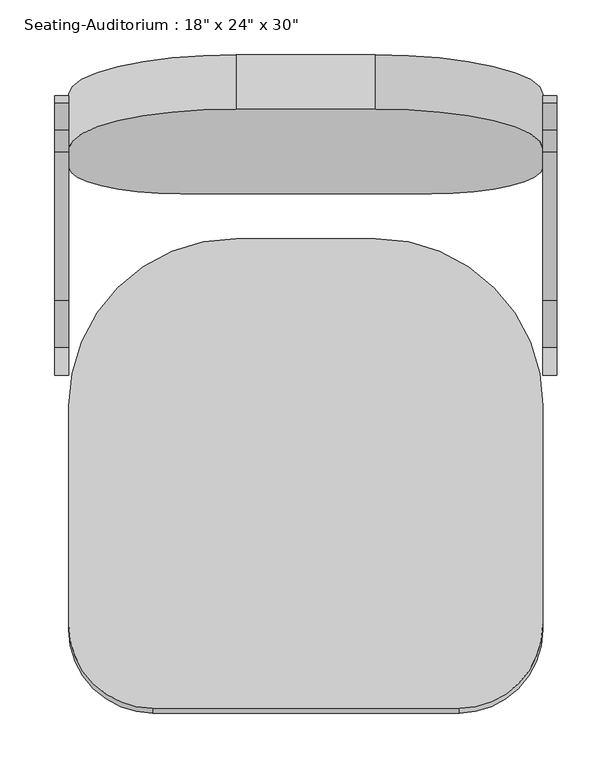
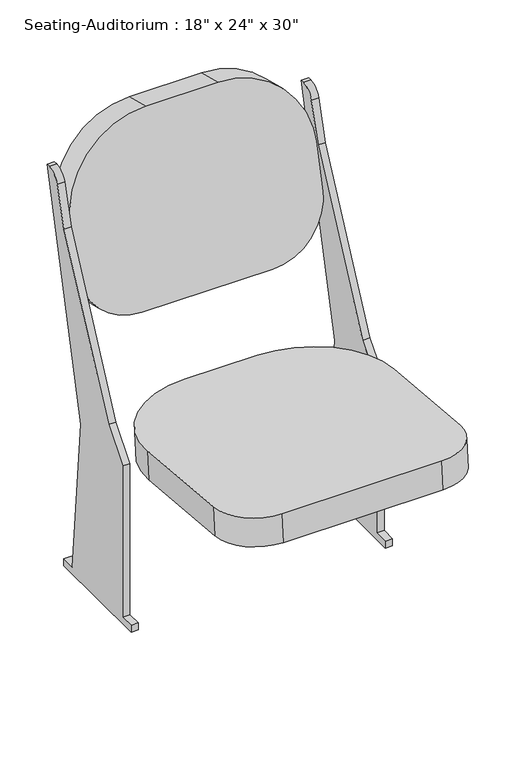
"""IFC4 building model written with IfcOpenShell, lengths in millimetres: furniture geometry."""

from ifc_helpers import new_model, si_unit, point, frame, frame_2d, origin, place, context, project, spatial, polyline, circle_curve, trimmed, segment, composite_curve, outline, extrude, source, transform, mapped, element, save


def furniture_4fdbbe14(model_context):
    return source(origin(), model_context, "Body", "SweptSolid", [
        extrude(outline(composite_curve([segment(polyline([(13.3245902, 12.7), (13.3245902, 0.0), (-189.8754098, 0.0), (-189.8754098, 12.7), (-164.4754098, 12.7), (-164.4754098, 292.1), (-121.8491486, 342.9), (13.3245902, 622.3), (33.4611378, 692.7779166)]), True, "CONTINUOUS"), segment(trimmed(circle_curve(frame_2d((57.883846, 685.8)), 25.4), [point((33.4611378, 692.7779166))], [point((57.883846, 711.2))], False, "CARTESIAN"), True, "CONTINUOUS"), segment(polyline([(57.883846, 711.2), (64.1245902, 711.2), (-37.4754098, 292.1), (-12.0754098, 12.7), (13.3245902, 12.7)]), True, "CONTINUOUS")], self_intersect=False)), frame((376.6278689, 0.0, 0.0), z_axis=(1.0, 0.0, 0.0), x_axis=(0.0, 1.0, 0.0)), (0.0, 0.0, 1.0), 12.7),
        extrude(outline(composite_curve([segment(polyline([(13.3245902, 0.0), (-189.8754098, 0.0), (-189.8754098, 12.7), (-164.4754098, 12.7), (-164.4754098, 292.1), (-121.8491486, 342.9), (13.3245902, 622.3), (33.4611378, 692.7779166)]), True, "CONTINUOUS"), segment(trimmed(circle_curve(frame_2d((57.883846, 685.8)), 25.4), [point((33.4611378, 692.7779166))], [point((57.883846, 711.2))], False, "CARTESIAN"), True, "CONTINUOUS"), segment(polyline([(57.883846, 711.2), (64.1245902, 711.2), (-37.4754098, 292.1), (-12.0754098, 12.7), (13.3245902, 12.7), (13.3245902, 0.0)]), True, "CONTINUOUS")], self_intersect=False)), frame((-67.8721311, 0.0, 0.0), z_axis=(1.0, 0.0, 0.0), x_axis=(0.0, 1.0, 0.0)), (0.0, 0.0, 1.0), 12.7),
        extrude(outline(composite_curve([segment(polyline([(0.0, 0.0), (-279.4, 0.0)]), True, "CONTINUOUS"), segment(trimmed(circle_curve(frame_2d((-279.4, 76.2)), 76.2), [point((-279.4, 0.0))], [point((-355.6, 76.2))], False, "CARTESIAN"), True, "CONTINUOUS"), segment(polyline([(-355.6, 76.2), (-355.6, 276.4123505)]), True, "CONTINUOUS"), segment(trimmed(circle_curve(frame_2d((-203.2, 276.4123505)), 152.4), [point((-355.6, 276.4123505))], [point((-203.2, 428.8123506))], False, "CARTESIAN"), True, "CONTINUOUS"), segment(polyline([(-203.2, 428.8123506), (-76.2, 428.8123506)]), True, "CONTINUOUS"), segment(trimmed(circle_curve(frame_2d((-76.2, 276.4123505)), 152.4), [point((-76.2, 428.8123506))], [point((76.2, 276.4123505))], False, "CARTESIAN"), True, "CONTINUOUS"), segment(polyline([(76.2, 276.4123505), (76.2, 76.2)]), True, "CONTINUOUS"), segment(trimmed(circle_curve(frame_2d((0.0, 76.2)), 76.2), [point((76.2, 76.2))], [point((0.0, 0.0))], False, "CARTESIAN"), True, "CONTINUOUS")], self_intersect=False)), frame((300.4278689, -497.5245173, 321.2380213), z_axis=(0.0, 0.08715574274765496, 0.9961946980917459), x_axis=(1.0, 0.0, 0.0)), (0.0, 0.0, 1.0), 50.8),
        extrude(outline(composite_curve([segment(trimmed(circle_curve(frame_2d((0.0, 152.4)), 152.4), [point((0.0, 0.0))], [point((-152.4, 152.4))], False, "CARTESIAN"), True, "CONTINUOUS"), segment(polyline([(-152.4, 152.4), (-152.4, 224.0588601)]), True, "CONTINUOUS"), segment(trimmed(circle_curve(frame_2d((-50.8, 224.0588601)), 101.6), [point((-152.4, 224.0588601))], [point((-50.8, 325.6588601))], False, "CARTESIAN"), True, "CONTINUOUS"), segment(polyline([(-50.8, 325.6588601), (177.8, 325.6588601)]), True, "CONTINUOUS"), segment(trimmed(circle_curve(frame_2d((177.8, 224.0588601)), 101.6), [point((177.8, 325.6588601))], [point((279.4, 224.0588601))], False, "CARTESIAN"), True, "CONTINUOUS"), segment(polyline([(279.4, 224.0588601), (279.4, 152.4)]), True, "CONTINUOUS"), segment(trimmed(circle_curve(frame_2d((127.0, 152.4)), 152.4), [point((279.4, 152.4))], [point((127.0, 0.0))], False, "CARTESIAN"), True, "CONTINUOUS"), segment(polyline([(127.0, 0.0), (0.0, 0.0)]), True, "CONTINUOUS")], self_intersect=False)), frame((224.2278689, 101.3396919, 755.9484479), z_axis=(0.0, -0.9717404775047361, 0.23605178325712217), x_axis=(-1.0, 0.0, 0.0)), (0.0, 0.0, 1.0), 50.8),
    ])


if __name__ == "__main__":
    model = new_model("IFC4")
    model_context = context("Model", 3, world=origin())
    ifc_project = project(units=[si_unit("LENGTHUNIT", "METRE", prefix="MILLI")], contexts=[model_context])
    site = spatial("IfcSite", under=ifc_project)
    building = spatial("IfcBuilding", under=site)
    placement = place(None, origin())
    furniture_shape = furniture_4fdbbe14(model_context)
    element("IfcFurniture", 1, ObjectType="Seating-Auditorium : 18\" x 24\" x 30\"", at=placement, inside=building, context=model_context, shape_type="MappedRepresentation", body=[
        mapped(furniture_shape, transform((0.0, 0.0, 0.0), x_axis=(1.0, 0.0, 0.0), y_axis=(0.0, 1.0, 0.0), z_axis=(0.0, 0.0, 1.0))),
    ])
    save(model, "model.ifc")

# Revit data of these elements
# Type "Seating-Auditorium : 18\" x 24\" x 30\""
#   Assembly Code = "E2020200"
#   Seat Material = Linen, Beige
#   Frame Material = Steel, Paint Finish, Dark Gray, Matte
#   Default Elevation = 0
# Element 1 (IfcFurniture, "Seating-Auditorium : 18\" x 24\" x 30\"")
#   Materials on its faces: "Steel, Paint Finish, Dark Gray, Matte", "Linen, Beige"
# Materials
#   "Linen, Beige": class "Textile", colour RGB 249 239 230, transparency 0, Description = "Linen, beige", Cost = 0
#   "Steel, Paint Finish, Dark Gray, Matte": class "Metal", colour RGB 0 0 0, transparency 0, Description = "Steel, paint finish, dark gray, matte", Cost = 0
